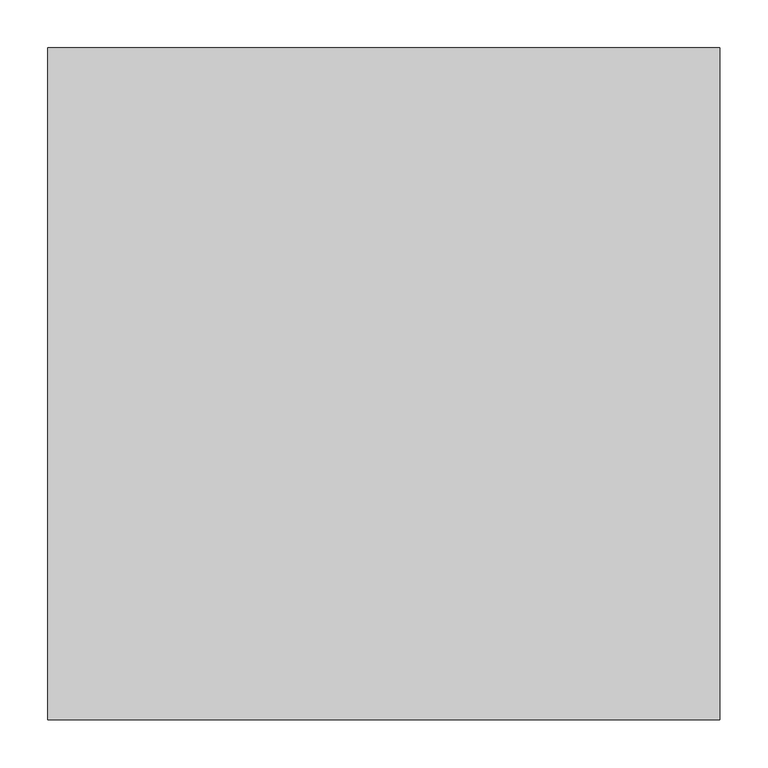
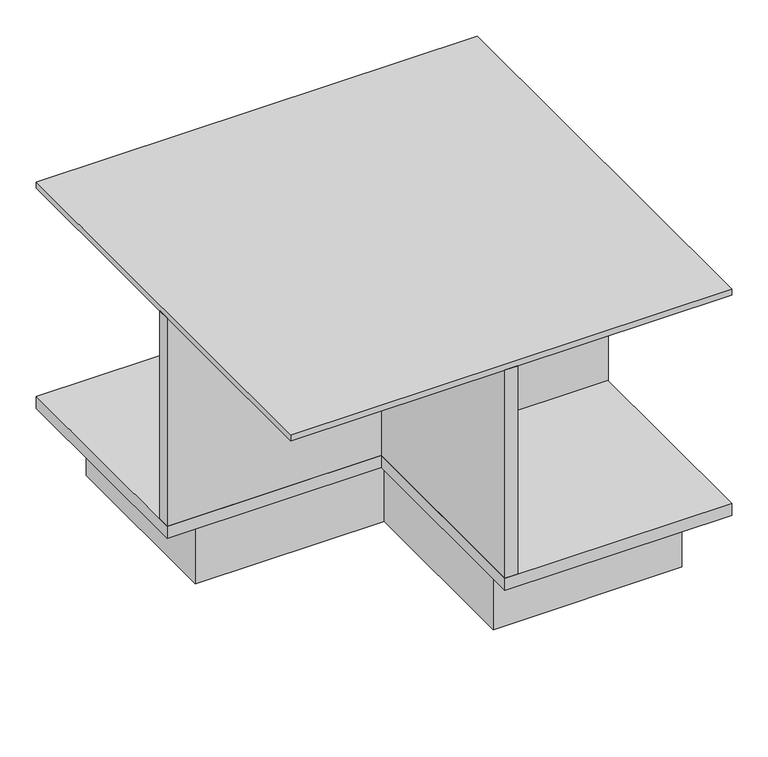
"""IFC4 building model written with IfcOpenShell, lengths in millimetres: furniture geometry."""

from ifc_helpers import new_model, si_unit, frame, origin, origin_with_axes, place, context, project, spatial, polyline, outline, extrude, source, transform, mapped, element, save


def furniture_061ed33e(model_context):
    return source(origin(), model_context, "Body", "SweptSolid", [
        extrude(outline(polyline([(-300.0, 0.0), (-300.0, 300.0), (0.0, 300.0), (0.0, 0.0), (-300.0, 0.0)])), origin_with_axes(), (0.0, 0.0, 1.0), 100.0),
        extrude(outline(polyline([(0.0, -300.0), (0.0, 0.0), (300.0, 0.0), (300.0, -300.0), (0.0, -300.0)])), origin_with_axes(), (0.0, 0.0, 1.0), 100.0),
        extrude(outline(polyline([(10.0, 350.0), (10.0, 10.0), (350.0, 10.0), (350.0, -350.0), (-10.0, -350.0), (-10.0, -10.0), (-350.0, -10.0), (-350.0, 350.0), (10.0, 350.0)])), frame((0.0, 0.0, 100.0), z_axis=(0.0, 0.0, 1.0), x_axis=(1.0, 0.0, 0.0)), (0.0, 0.0, 1.0), 20.0),
        extrude(outline(polyline([(-10.0, 10.0), (-10.0, 350.0), (10.0, 350.0), (10.0, 10.0), (350.0, 10.0), (350.0, -10.0), (10.0, -10.0), (10.0, -350.0), (-10.0, -350.0), (-10.0, -10.0), (-350.0, -10.0), (-350.0, 10.0), (-10.0, 10.0)])), frame((0.0, 0.0, 120.0), z_axis=(0.0, 0.0, 1.0), x_axis=(1.0, 0.0, 0.0)), (0.0, 0.0, 1.0), 350.0),
        extrude(outline(polyline([(350.0, 350.0), (350.0, -350.0), (-350.0, -350.0), (-350.0, 350.0), (350.0, 350.0)])), frame((0.0, 0.0, 470.0), z_axis=(0.0, 0.0, 1.0), x_axis=(1.0, 0.0, 0.0)), (0.0, 0.0, 1.0), 10.0),
    ])


if __name__ == "__main__":
    model = new_model("IFC4")
    model_context = context("Model", 3, world=origin())
    ifc_project = project(units=[si_unit("LENGTHUNIT", "METRE", prefix="MILLI")], contexts=[model_context])
    site = spatial("IfcSite", under=ifc_project)
    building = spatial("IfcBuilding", under=site)
    placement = place(None, origin())
    furniture_shape = furniture_061ed33e(model_context)
    element("IfcFurniture", 1, at=placement, inside=building, context=model_context, shape_type="MappedRepresentation", body=[
        mapped(furniture_shape, transform((0.0, 0.0, 0.0), x_axis=(1.0, 0.0, 0.0), y_axis=(0.0, 1.0, 0.0), z_axis=(0.0, 0.0, 1.0))),
    ])
    save(model, "model.ifc")

# Revit data of these elements
# Type
#   Default Elevation = 0
# Element 1 (IfcFurniture)
#   Materials on its faces: "Wood", "0 Glass"
# Materials
#   "Wood": class "Wood", colour RGB 212 179 113, transparency 0, Description = "Generic wood", Cost = 0
#   "0 Glass": colour RGB 243 243 243, transparency 0.92
